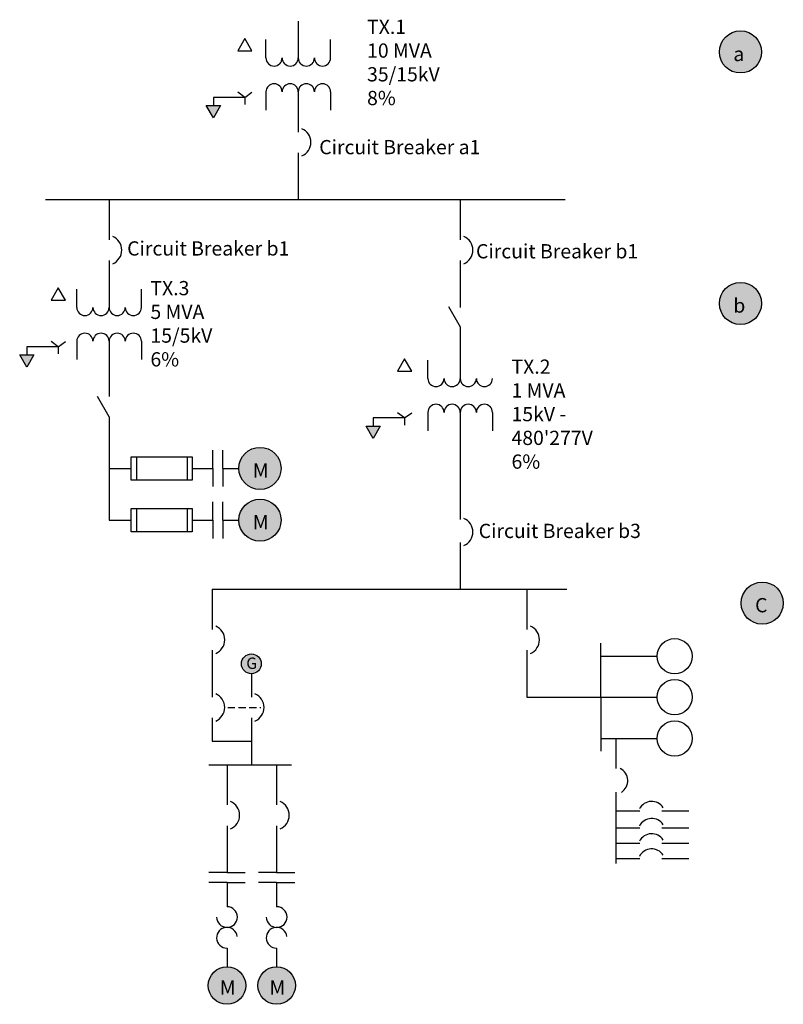
# Model space of a CAD drawing. Units: millimetres. Extents: x 55.4 to 109, y 5.9 to 75.
import ezdxf

# ---------------------------------------------------------------- set-up
doc = ezdxf.new("R2010")
doc.units = ezdxf.units.MM
doc.header["$MEASUREMENT"] = 0
doc.linetypes.add('HIDDENX2', pattern=[0.75, 0.5, -0.25])
for name, color, linetype, lineweight in [('E-ANNO-IDEN', 250, 'Continuous', 30), ('E-ANNO-SYMB', 7, 'Continuous', 30), ('E-ANNO-SYMB-PATT', 9, 'Continuous', 30), ('E-ANNO-TEXT', 7, 'Continuous', 30), ('E-POWR-BUSB', 1, 'Continuous', 30), ('E-POWR-CONN', 7, 'Continuous', 30), ('E-POWR-FEED', 7, 'Continuous', 25), ('E-POWR-GENR', 7, 'Continuous', 30), ('E-POWR-INTL', 7, 'HIDDENX2', 30), ('E-POWR-LOAD', 7, 'Continuous', 30), ('E-POWR-MOTR', 7, 'Continuous', 30), ('E-POWR-MOTR-PATT', 4, 'Continuous', 30), ('E-POWR-PROT', 7, 'Continuous', 30), ('E-POWR-SWGR', 7, 'Continuous', 25), ('E-POWR-XFMR', 7, 'Continuous', 25)]:
    doc.layers.add(name, color=color, linetype=linetype, lineweight=lineweight)
doc.layers.add('E-POWR-GENR-PATT', color=114, linetype='Continuous', lineweight=30, true_color=0x139b48)
doc.layers.add('E-POWR-GRND-PATT', color=18, linetype='Continuous', lineweight=30, true_color=0x000000)
doc.styles.get("Standard").update_dxf_attribs({"font": 'arial.ttf'})

# ---------------------------------------------------------------- blocks, each defined once
blk = doc.blocks.new('XFMR-TWO-WINDING')
for p, q in [((-2.268, 0), (-2.268, 1.291)), ((2.268, 0), (2.268, 1.291)), ((-2.268, -2.377), (-2.268, -3.667)), ((2.268, -2.377), (2.268, -3.667))]:
    blk.add_line(p, q)
for centre, start, end in [((-1.701, 0), 180, 0), ((-0.567, 0), 180, 0), ((0.567, 0), 180, 0), ((1.701, 0), 180, 0), ((-1.701, -2.377), 0, 180), ((-0.567, -2.377), 0, 180), ((0.567, -2.377), 0, 180), ((1.701, -2.377), 0, 180)]:
    blk.add_arc(centre, 0.567, start, end)
blk = doc.blocks.new('CB-INLINE')
for p, q in [((0, 0), (0, -2.828)), ((0, -4.283), (0, -7.571))]:
    blk.add_line(p, q)
blk.add_arc((-0.15, -3.546), 1.038, 292.81895, 67.18105)
blk = doc.blocks.new('CB-BRANCH')
for p, q in [((0, 0), (1.682, 0)), ((3.237, 0), (5.129, 0))]:
    blk.add_line(p, q)
blk.add_arc((2.517, -0.306), 0.972, 33.05277, 153.05277)
blk = doc.blocks.new('FUSE-CARTRIDGE')
for p, q in [((0.359, 0.815), (0.359, -0.815)), ((3.932, 0.815), (3.932, -0.815))]:
    blk.add_line(p, q)
blk.add_lwpolyline([(0, 0.815), (4.281, 0.815), (4.281, -0.815), (0, -0.815)], close=True)
blk = doc.blocks.new('CONTACT-NO')
for p, q in [((0, 0), (0, 1.281)), ((0.703, 0), (0.703, 1.281)), ((0, 0), (0, -1.281)), ((0.703, 0), (0.703, -1.281))]:
    blk.add_line(p, q)
blk = doc.blocks.new('MOTOR-OVERLOAD')
for centre, start, end in [((0, -0.729), 180.77364, 90), ((0, -2.187), 7.26928, 270)]:
    blk.add_arc(centre, 0.729, start, end)
blk = doc.blocks.new('LOAD-TERMINAL')
blk.add_line((0, 0), (3.94, 0))
blk.add_circle((5.176, 0), 1.235)
blk = doc.blocks.new('DISCONNECT-BLADE')
blk.add_line((0, 0), (-0.823, 1.426))
blk = doc.blocks.new('XFMR-DELTA')
blk.add_lwpolyline([(0, 0), (-0.499, -0.864), (0.499, -0.864)], close=True)
blk = doc.blocks.new('XFMR-GROUNDED-WYE')
for p, q in [((0, 0), (-2.208, 0)), ((0, 0), (-0.499, 0.366)), ((0, 0), (0.499, 0.366)), ((0, 0), (0, -0.499)), ((-2.208, 0), (-2.208, -0.569))]:
    blk.add_line(p, q)

msp = doc.modelspace()

# ---------------------------------------------------------------- hatches: boundary and pattern name
at = {"layer": 'E-ANNO-SYMB-PATT'}
h = msp.add_hatch(color=256, dxfattribs=at)
h.dxf.hatch_style = 1
h.paths.add_polyline_path([(104.525, 72.782, 1), (107.485, 72.782, 1)])
h = msp.add_hatch(color=256, dxfattribs=at)
h.dxf.hatch_style = 1
h.paths.add_polyline_path([(107.485, 55.117, 1), (104.525, 55.117, 1)])
h = msp.add_hatch(color=256, dxfattribs=at)
h.dxf.hatch_style = 1
h.paths.add_polyline_path([(106.053, 34.072, 1), (109.013, 34.072, 1)])
at = {"layer": 'E-POWR-GENR-PATT'}
h = msp.add_hatch(color=256, dxfattribs=at)
h.dxf.hatch_style = 1
h.paths.add_polyline_path([(70.969, 29.81, 1), (72.361, 29.81, 1)])
at = {"layer": 'E-POWR-GRND-PATT'}
h = msp.add_hatch(color=256, dxfattribs=at)
h.dxf.hatch_style = 1
h.paths.add_polyline_path([(69.495, 69.019), (68.497, 69.019), (68.996, 68.155)])
h = msp.add_hatch(color=256, dxfattribs=at)
h.dxf.hatch_style = 1
h.paths.add_polyline_path([(56.398, 51.5), (55.4, 51.5), (55.899, 50.635)])
h = msp.add_hatch(color=256, dxfattribs=at)
h.dxf.hatch_style = 1
h.paths.add_polyline_path([(80.718, 46.507), (79.72, 46.507), (80.219, 45.643)])
at = {"layer": 'E-POWR-MOTR-PATT'}
h = msp.add_hatch(color=256, dxfattribs=at)
h.dxf.hatch_style = 1
h.paths.add_polyline_path([(73.749, 43.532, 1), (70.789, 43.532, 1)])
h.paths.add_polyline_path([(73.749, 39.899, 1), (70.789, 39.899, 1)])
h.paths.add_polyline_path([(71.273, 7.215, 1), (68.637, 7.215, 1)])
h.paths.add_polyline_path([(74.758, 7.215, 1), (72.122, 7.215, 1)])

# ---------------------------------------------------------------- linework, layer by layer
at = {"layer": 'E-ANNO-SYMB'}
for centre in [(106.005, 72.782), (106.005, 55.117), (107.533, 34.072)]:
    msp.add_circle(centre, 1.48, dxfattribs=at)
at = {"layer": 'E-POWR-BUSB'}
for p, q in [((57.216, 62.409), (93.701, 62.409)), ((68.909, 35.041), (93.823, 35.041)), ((68.691, 22.724), (74.494, 22.724))]:
    msp.add_line(p, q, dxfattribs=at)
at = {"layer": 'E-POWR-CONN'}
for points in [[(68.497, 69.019), (69.495, 69.019), (68.996, 68.155)], [(55.4, 51.5), (56.398, 51.5), (55.899, 50.635)], [(79.72, 46.507), (80.718, 46.507), (80.219, 45.643)]]:
    msp.add_lwpolyline(points, close=True, dxfattribs=at)
at = {"layer": 'E-POWR-FEED'}
for p, q in [((74.959, 74.938), (74.959, 72.357)), ((86.327, 53.478), (86.327, 49.845)), ((61.678, 52.461), (61.678, 49.633)), ((61.678, 49.633), (61.678, 48.59)), ((61.678, 47.164), (61.678, 39.899)), ((86.327, 47.468), (86.327, 44.64)), ((86.327, 47.468), (86.327, 39.934)), ((61.678, 43.532), (63.234, 43.532)), ((67.515, 43.532), (68.964, 43.532)), ((69.667, 43.532), (70.789, 43.532)), ((61.678, 39.899), (63.234, 39.899)), ((67.515, 39.899), (68.964, 39.899)), ((69.667, 39.899), (70.789, 39.899)), ((86.327, 38.33), (86.327, 35.041)), ((96.213, 27.469), (96.213, 31.254)), ((71.665, 29.114), (71.665, 27.469)), ((91.004, 27.469), (96.213, 27.469)), ((96.213, 27.469), (96.213, 23.685)), ((68.909, 26.013), (68.909, 24.369)), ((71.665, 26.013), (71.665, 22.724)), ((68.909, 24.369), (71.665, 24.369)), ((97.257, 24.567), (97.257, 22.465)), ((97.257, 20.784), (97.257, 15.785)), ((69.955, 14.45), (69.955, 12.754)), ((73.44, 14.45), (73.44, 12.754)), ((69.955, 9.838), (69.955, 8.533)), ((73.44, 9.838), (73.44, 8.533))]:
    msp.add_line(p, q, dxfattribs=at)
at = {"layer": 'E-POWR-GENR'}
msp.add_circle((71.665, 29.81), 0.696, dxfattribs=at)
at = {"layer": 'E-POWR-INTL'}
msp.add_line((70.016, 26.749), (72.335, 26.749), dxfattribs=at)
at = {"layer": 'E-POWR-MOTR'}
for centre, radius in [((72.269, 43.532), 1.48), ((72.269, 39.899), 1.48), ((69.955, 7.215), 1.318), ((73.44, 7.215), 1.318)]:
    msp.add_circle(centre, radius, dxfattribs=at)
at = {"layer": 'E-POWR-SWGR'}
for centre, radius, start, end in [((86.177, 39.066), 1.038, 292.81895, 67.18105), ((68.758, 26.749), 1.038, 292.81895, 67.18105), ((71.515, 26.749), 1.038, 292.81895, 67.18105), ((97.117, 21.598), 0.972, 303.05277, 63.05277)]:
    msp.add_arc(centre, radius, start, end, dxfattribs=at)
at = {"layer": 'E-POWR-XFMR'}
for p, q in [((84.059, 49.845), (84.059, 51.136)), ((84.059, 47.468), (84.059, 46.178)), ((88.595, 47.468), (88.595, 46.178))]:
    msp.add_line(p, q, dxfattribs=at)
for centre, start, end in [((84.626, 49.845), 180, 0), ((85.76, 49.845), 180, 0), ((86.894, 49.845), 180, 0), ((88.028, 49.845), 180, 0), ((84.626, 47.468), 0, 180), ((85.76, 47.468), 0, 180), ((86.894, 47.468), 0, 180), ((88.028, 47.468), 0, 180)]:
    msp.add_arc(centre, 0.567, start, end, dxfattribs=at)

# ---------------------------------------------------------------- block references
at = {"layer": 'E-POWR-CONN'}
for name, p in [('XFMR-DELTA', (71.204, 73.731)), ('XFMR-GROUNDED-WYE', (71.204, 69.588)), ('XFMR-DELTA', (58.107, 56.212)), ('XFMR-GROUNDED-WYE', (58.107, 52.069)), ('XFMR-DELTA', (82.427, 51.219)), ('XFMR-GROUNDED-WYE', (82.427, 47.076))]:
    msp.add_blockref(name, p, dxfattribs=at)
at = {"layer": 'E-POWR-LOAD'}
for p in [(96.213, 30.344), (96.213, 27.469), (96.213, 24.567)]:
    msp.add_blockref('LOAD-TERMINAL', p, dxfattribs=at)
at = {"layer": 'E-POWR-PROT'}
for name, p in [('FUSE-CARTRIDGE', (63.234, 43.532)), ('FUSE-CARTRIDGE', (63.234, 39.899)), ('MOTOR-OVERLOAD', (69.955, 12.754)), ('MOTOR-OVERLOAD', (73.44, 12.754))]:
    msp.add_blockref(name, p, dxfattribs=at)
at = {"layer": 'E-POWR-SWGR'}
for name, p in [('CB-INLINE', (74.959, 69.98)), ('CB-INLINE', (61.678, 62.409)), ('CB-INLINE', (86.327, 62.409)), ('DISCONNECT-BLADE', (61.678, 47.164)), ('CONTACT-NO', (68.964, 43.532)), ('CONTACT-NO', (68.964, 39.899)), ('CB-INLINE', (68.909, 35.041)), ('CB-INLINE', (91.004, 35.041)), ('CB-INLINE', (69.955, 22.724)), ('CB-INLINE', (73.44, 22.724)), ('CB-BRANCH', (97.257, 19.482)), ('CB-BRANCH', (97.257, 18.285)), ('CB-BRANCH', (97.257, 17.21)), ('CB-BRANCH', (97.257, 16.145))]:
    msp.add_blockref(name, p, dxfattribs=at)
for name, p, rotation in [('DISCONNECT-BLADE', (85.504, 54.903), 180), ('CONTACT-NO', (69.955, 14.45), 90.00000000000006), ('CONTACT-NO', (73.44, 14.45), 90.00000000000006)]:
    msp.add_blockref(name, p, dxfattribs=dict(at, rotation=rotation))
at = {"layer": 'E-POWR-XFMR'}
for p in [(74.959, 72.357), (61.678, 54.838)]:
    msp.add_blockref('XFMR-TWO-WINDING', p, dxfattribs=at)

# ---------------------------------------------------------------- texts
at = {"layer": 'E-ANNO-IDEN', "attachment_point": 1}
for s, width, insert, char_height in [('a', 0.50202, (105.503, 73.136), 1), ('b', 0.50202, (105.503, 55.472), 1), ('M', 0.50202, (71.767, 43.886), 1), ('M', 0.50202, (71.767, 40.254), 1), ('C', 1, (107.031, 34.427), 1), ('G', 0.50202, (71.309, 30.249), 0.8), ('M', 0.50202, (69.453, 7.57), 1), ('M', 0.50202, (72.938, 7.57), 1)]:
    msp.add_mtext_dynamic_manual_height_columns(s, width=width, gutter_width=1, heights=[0], dxfattribs=dict(at, insert=insert, char_height=char_height))
at = {"layer": 'E-ANNO-TEXT', "char_height": 1, "attachment_point": 1}
for s, width, insert in [('TX.1\\P10 MVA\\P35/15kV\\P8%', 7.48842, (79.79, 75.045)), ('Circuit Breaker a1', 11.79872, (76.431, 66.596)), ('Circuit Breaker b1', 11.79872, (62.944, 59.48)), ('Circuit Breaker b1', 11.79872, (87.437, 59.284)), ('TX.3\\P5 MVA\\P15/5kV\\P6%', 7.48842, (64.579, 56.694)), ("TX.2\\P1 MVA\\P15kV - 480'277V\\P6%", 7.48842, (89.931, 51.178)), ('Circuit Breaker b3', 11.79872, (87.626, 39.643))]:
    msp.add_mtext_dynamic_manual_height_columns(s, width=width, gutter_width=1, heights=[0], dxfattribs=dict(at, insert=insert))

doc.saveas('drawing.dxf')
